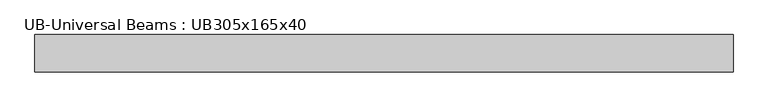
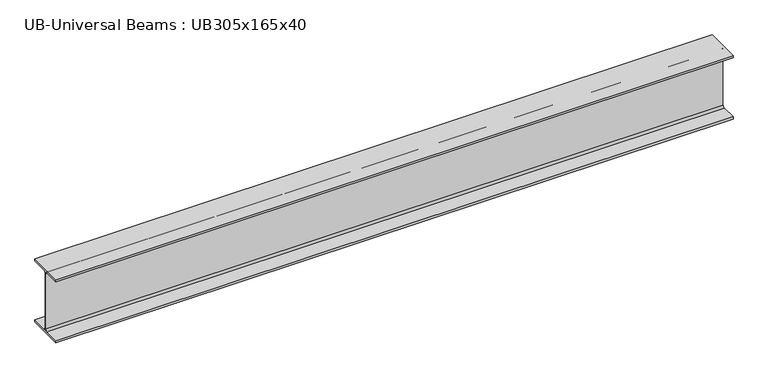
"""IFC4 building model written with IfcOpenShell, lengths in millimetres: beam geometry, UB-Universal Beams : UB305x165x40."""

from ifc_helpers import new_model, si_unit, point, frame, frame_2d, origin, place, context, project, spatial, polyline, circle_curve, trimmed, segment, composite_curve, outline, extrude, source, transform, mapped, element, save


def ub_universal_beams_ub305x165x40_603755b3(model_context):
    return source(origin(), model_context, "Body", "SweptSolid", [
        extrude(outline(composite_curve([segment(polyline([(82.5, -141.5), (82.5, -151.7), (-82.5, -151.7), (-82.5, -141.5), (-11.9, -141.5)]), True, "CONTINUOUS"), segment(trimmed(circle_curve(frame_2d((-11.9, -132.6)), 8.9), [point((-11.9, -141.5))], [point((-3.0, -132.6))], True, "CARTESIAN"), True, "CONTINUOUS"), segment(polyline([(-3.0, -132.6), (-3.0, 132.6)]), True, "CONTINUOUS"), segment(trimmed(circle_curve(frame_2d((-11.9, 132.6)), 8.9), [point((-3.0, 132.6))], [point((-11.9, 141.5))], True, "CARTESIAN"), True, "CONTINUOUS"), segment(polyline([(-11.9, 141.5), (-82.5, 141.5), (-82.5, 151.7), (82.5, 151.7), (82.5, 141.5), (11.9, 141.5)]), True, "CONTINUOUS"), segment(trimmed(circle_curve(frame_2d((11.9, 132.6)), 8.9), [point((11.9, 141.5))], [point((3.0, 132.6))], True, "CARTESIAN"), True, "CONTINUOUS"), segment(polyline([(3.0, 132.6), (3.0, -132.6)]), True, "CONTINUOUS"), segment(trimmed(circle_curve(frame_2d((11.9, -132.6)), 8.9), [point((3.0, -132.6))], [point((11.9, -141.5))], True, "CARTESIAN"), True, "CONTINUOUS"), segment(polyline([(11.9, -141.5), (82.5, -141.5)]), True, "CONTINUOUS")], self_intersect=False)), frame((-1487.2, 0.0, 0.0), z_axis=(1.0, 0.0, 0.0), x_axis=(0.0, 1.0, 0.0)), (0.0, 0.0, 1.0), 3069.7),
    ])


if __name__ == "__main__":
    model = new_model("IFC4")
    model_context = context("Model", 3, world=origin())
    ifc_project = project(units=[si_unit("LENGTHUNIT", "METRE", prefix="MILLI")], contexts=[model_context])
    site = spatial("IfcSite", under=ifc_project)
    building = spatial("IfcBuilding", under=site)
    placement = place(None, origin())
    ub_universal_beams_ub305x165x40_shape = ub_universal_beams_ub305x165x40_603755b3(model_context)
    element("IfcBeam", 1, ObjectType="UB-Universal Beams : UB305x165x40", at=placement, inside=building, context=model_context, shape_type="MappedRepresentation", body=[
        mapped(ub_universal_beams_ub305x165x40_shape, transform((0.0, 0.0, 0.0), x_axis=(1.0, 0.0, 0.0), y_axis=(0.0, 1.0, 0.0), z_axis=(0.0, 0.0, 1.0))),
    ])
    save(model, "model.ifc")

# Revit data of these elements
# Type "UB-Universal Beams : UB305x165x40"
#   Section Name Key = "UB305X165X40"
#   Width = 16.5 cm
#   Web Thickness = 0.6 cm
#   Web Fillet = 0.89 cm
#   Warping Constant = 164000.0 cm⁶
#   Torsional Moment of Inertia = 14.70 cm⁴
#   Section Area = 51.3 cm²
#   Plastic Modulus weak axis = 142.0 cm³
#   Plastic Modulus strong axis = 623.0 cm³
#   Nominal Weight = 40.2999 kgf/m
#   Moment of Inertia weak axis = 764.00 cm⁴
#   Moment of Inertia strong axis = 8503.00 cm⁴
#   Height = 30.34 cm
#   Flange Thickness = 1.02 cm
#   Elastic Modulus weak axis = 92.6 cm³
#   Elastic Modulus strong axis = 560.0 cm³
#   Centroid Vertical = 15.17 cm
#   Centroid Horizontal = 8.25 cm
#   Bolt Spacing = 9.0 cm
#   Length [instance default] = 1.5 m
#   Structural Material [instance default] = Metal - Steel 43-275
#   Type Comments = ""
#   Assembly Code = ""
# Element 1 (IfcBeam, "UB-Universal Beams : UB305x165x40")
#   Materials on its faces: "Metal - Steel 43-275"
# Materials
#   "Metal - Steel 43-275": class "Metal", colour RGB 247 247 247, transparency 0, Cost = 0
